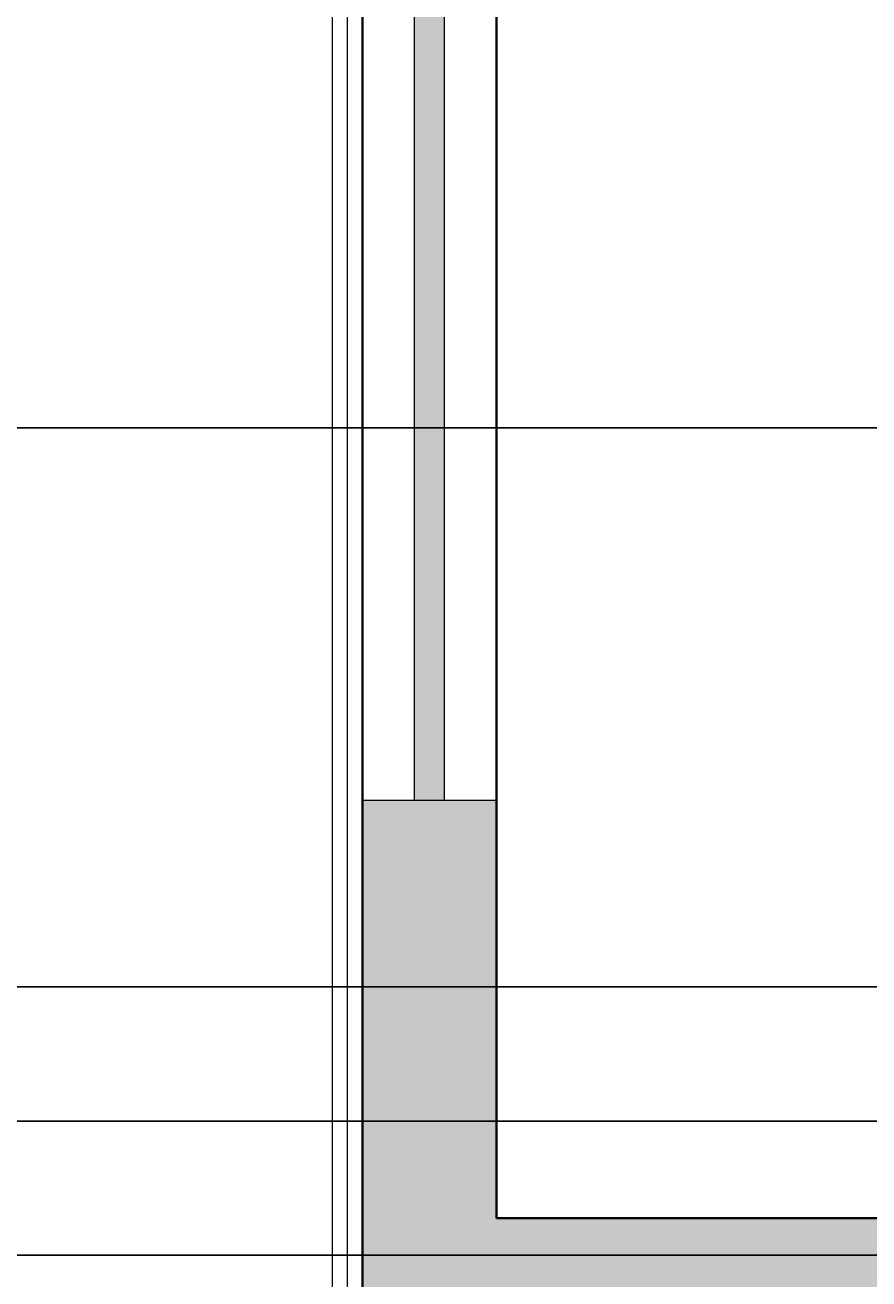
# Model space of a CAD drawing. Units: inches. Extents: x 311 to 815, y -527 to 136.
# Tile 7 of 21: x 388 to 444, y -294 to -210. Entities that reach past the tile are written whole.
import ezdxf

# ---------------------------------------------------------------- set-up
doc = ezdxf.new("R2010")
doc.units = ezdxf.units.IN
doc.header["$MEASUREMENT"] = 0
for name, color, linetype, lineweight in [('A-ANNO-DIMS', 1, 'Continuous', 18), ('A-FLOR-EDGE', 1, 'Continuous', 18), ('A-GLAZ-PATT', 5, 'Continuous', 13), ('A-WALL-PATT', 242, 'Continuous', 13), ('wall', 1, 'Continuous', 35), ('win', 5, 'Continuous', 18)]:
    doc.layers.add(name, color=color, linetype=linetype, lineweight=lineweight)
doc.styles.get("Standard").update_dxf_attribs({"font": 'arial.ttf'})
doc.dimstyles.get("Standard").update_dxf_attribs({"dimtxt": 0.18, "dimasz": 0.18, "dimexe": 0.18, "dimexo": 0.0625, "dimgap": 0.09, "dimtad": 0, "dimtih": 1, "dimtoh": 1, "dimdec": 1, "dimzin": 0, "dimdsep": 46, "dimlunit": 4, "dimtxsty": 'Standard', "dimcen": 0.09, "dimadec": 0, "dimazin": 0, "dimtfac": 1, "dimtdec": 1, "dimtofl": 0, "dimtmove": 0, "dimatfit": 3, "dimfxl": 1, "dimtolj": 1, "dimtzin": 0, "dimarcsym": 0})

# ---------------------------------------------------------------- blocks, each defined once
blk = doc.blocks.new('_ArchTick')
at = {"color": 0, "linetype": 'ByBlock', "const_width": 0.15}
blk.add_lwpolyline([(-0.5, -0.5), (0.5, 0.5)], dxfattribs=at)
blk = doc.blocks.new('_Oblique')
at = {"color": 0, "linetype": 'ByBlock', "lineweight": -2}
blk.add_line((-0.5, -0.5), (0.5, 0.5), dxfattribs=at)
blk = doc.blocks.new('*D3')
at = {"layer": 'A-ANNO-DIMS', "color": 0, "lineweight": -2, "transparency": 16777216}
for p, q in [((377.538, 21.872), (377.538, -221.609)), ((377.538, -482.128), (377.538, -238.646))]:
    blk.add_line(p, q, dxfattribs=at)
at = {"layer": 'Defpoints', "color": 0, "transparency": 16777216}
for p in [(410.323, 21.872), (377.538, -482.128), (410.323, -482.128)]:
    blk.add_point(p, dxfattribs=at)
at = {"layer": 'A-ANNO-DIMS', "color": 0, "lineweight": -2, "transparency": 16777216, "xscale": 9, "yscale": 9, "zscale": 9}
for name, p, rotation in [('_ArchTick', (377.538, 21.872), 90), ('_Oblique', (377.538, -482.128), 270)]:
    blk.add_blockref(name, p, dxfattribs=dict(at, rotation=rotation))
at = {"layer": 'A-ANNO-DIMS', "color": 0, "transparency": 16777216, "insert": (377.538, -230.128), "char_height": 9, "attachment_point": 5}
blk.add_mtext("\\A1;42'", dxfattribs=at)
blk = doc.blocks.new('WIN-60IN')
for p, q in [((9, 60), (0, 60)), ((3.5, 0), (3.5, 60)), ((5.5, 0), (5.5, 60)), ((9, 0), (0, 0))]:
    blk.add_line(p, q)
blk = doc.blocks.new('*D33')
at = {"layer": 'A-ANNO-DIMS', "color": 0, "lineweight": -2, "transparency": 16777216}
for p, q in [((609.26, -237.128), (377.793, -237.128)), ((377.973, -237.308), (377.973, -255.695)), ((377.973, -274.448), (377.973, -256.061)), ((609.26, -274.628), (377.793, -274.628))]:
    blk.add_line(p, q, dxfattribs=at)
at = {"layer": 'A-ANNO-DIMS', "color": 0, "transparency": 16777216}
for points in [[(377.943, -237.308), (378.003, -237.308), (377.973, -237.128)], [(377.943, -274.448), (378.003, -274.448), (377.973, -274.628)]]:
    blk.add_solid(points, dxfattribs=at)
at = {"layer": 'Defpoints', "color": 0, "transparency": 16777216}
for p in [(609.323, -237.128), (377.973, -274.628), (609.323, -274.628)]:
    blk.add_point(p, dxfattribs=at)
at = {"layer": 'A-ANNO-DIMS', "color": 0, "transparency": 16777216, "insert": (377.973, -255.878), "char_height": 0.18, "attachment_point": 5}
blk.add_mtext('\\A1;3\'-1 1/2"', dxfattribs=at)
blk = doc.blocks.new('*D36')
at = {"layer": 'A-ANNO-DIMS', "color": 0, "lineweight": -2, "transparency": 16777216}
for p, q in [((665.26, -283.628), (377.793, -283.628)), ((377.973, -283.808), (377.973, -287.946)), ((377.973, -292.448), (377.973, -288.31)), ((665.26, -292.628), (377.793, -292.628))]:
    blk.add_line(p, q, dxfattribs=at)
at = {"layer": 'A-ANNO-DIMS', "color": 0, "transparency": 16777216}
for points in [[(377.943, -283.808), (378.003, -283.808), (377.973, -283.628)], [(377.943, -292.448), (378.003, -292.448), (377.973, -292.628)]]:
    blk.add_solid(points, dxfattribs=at)
at = {"layer": 'Defpoints', "color": 0, "transparency": 16777216}
for p in [(665.323, -283.628), (377.973, -292.628), (665.323, -292.628)]:
    blk.add_point(p, dxfattribs=at)
at = {"layer": 'A-ANNO-DIMS', "color": 0, "transparency": 16777216, "insert": (377.973, -288.128), "char_height": 0.18, "attachment_point": 5}
blk.add_mtext('\\A1;0\'-9"', dxfattribs=at)

msp = doc.modelspace()

# ---------------------------------------------------------------- hatches: boundary and pattern name
at = {"layer": 'A-GLAZ-PATT'}
h = msp.add_hatch(color=256, dxfattribs=at)
h.dxf.hatch_style = 1
h.paths.add_polyline_path([(415.823, -202.128), (413.823, -202.128), (413.823, -262.128), (415.823, -262.128)])
h.paths.add_polyline_path([(415.823, -390.84), (413.823, -390.84), (413.823, -450.84), (415.823, -450.84)])
h.paths.add_polyline_path([(415.823, -311.568), (413.823, -311.568), (413.823, -335.568), (415.823, -335.568)])
h.paths.add_polyline_path([(509.323, -476.628), (449.323, -476.628), (449.323, -478.628), (509.323, -478.628)])
h.paths.add_polyline_path([(606.823, -476.628), (582.823, -476.628), (582.823, -478.628), (606.823, -478.628)])
h.paths.add_polyline_path([(678.823, -476.628), (654.823, -476.628), (654.823, -478.628), (678.823, -478.628)])
h.paths.add_polyline_path([(718.823, -385.128), (716.823, -385.128), (716.823, -445.128), (718.823, -445.128)])
h.paths.add_polyline_path([(718.823, -262.628), (716.823, -262.628), (716.823, -322.628), (718.823, -322.628)])
h.paths.add_polyline_path([(718.823, -140.128), (716.823, -140.128), (716.823, -200.128), (718.823, -200.128)])
h.paths.add_polyline_path([(718.823, -18.128), (716.823, -18.128), (716.823, -42.128), (718.823, -42.128)])
h.paths.add_polyline_path([(686.823, 18.372), (626.823, 18.372), (626.823, 16.372), (686.823, 16.372)])
h.paths.add_polyline_path([(581.823, 18.372), (557.823, 18.372), (557.823, 16.372), (581.823, 16.372)])
h.paths.add_polyline_path([(509.323, 18.372), (449.323, 18.372), (449.323, 16.372), (509.323, 16.372)])
at = {"layer": 'A-WALL-PATT'}
h = msp.add_hatch(color=256, dxfattribs=at)
h.dxf.hatch_style = 1
h.paths.add_polyline_path([(557.823, 21.872), (509.323, 21.872), (509.323, 12.872), (539.323, 12.872), (539.323, -112.128), (548.323, -112.128), (548.323, -58.628), (557.823, -58.628), (557.823, -49.628), (548.323, -49.628), (548.323, 12.872), (557.823, 12.872)])
h.paths.add_polyline_path([(449.323, 21.872), (410.323, 21.872), (410.323, -15.128), (419.323, -15.128), (419.323, 12.872), (449.323, 12.872)])
h.paths.add_polyline_path([(626.823, 21.872), (581.823, 21.872), (581.823, 12.872), (591.323, 12.872), (591.323, -49.628), (581.823, -49.628), (581.823, -58.628), (591.323, -58.628), (591.323, -112.128), (600.323, -112.128), (600.323, 12.872), (626.823, 12.872)])
h.paths.add_polyline_path([(722.323, 21.872), (686.823, 21.872), (686.823, 12.872), (713.323, 12.872), (713.323, -18.128), (722.323, -18.128)])
h.paths.add_polyline_path([(722.323, -42.128), (713.323, -42.128), (713.323, -73.128), (722.323, -73.128)])
h.paths.add_polyline_path([(501.323, -103.128), (419.323, -103.128), (419.323, -75.128), (410.323, -75.128), (410.323, -126.628), (419.323, -126.628), (419.323, -112.128), (492.323, -112.128), (492.323, -143.128), (501.323, -143.128)])
h.paths.add_polyline_path([(548.323, -165.128), (419.323, -165.128), (419.323, -150.628), (410.323, -150.628), (410.323, -202.128), (419.323, -202.128), (419.323, -174.128), (548.323, -174.128)])
h.paths.add_polyline_path([(722.323, -103.128), (636.323, -103.128), (636.323, -112.128), (713.323, -112.128), (713.323, -140.128), (722.323, -140.128)])
h.paths.add_polyline_path([(548.323, -210.128), (539.323, -210.128), (539.323, -290.128), (419.323, -290.128), (419.323, -262.128), (410.323, -262.128), (410.323, -311.568), (419.323, -311.568), (419.323, -299.128), (469.323, -299.128), (469.323, -348.128), (443.323, -348.128), (443.323, -357.128), (478.323, -357.128), (478.323, -299.128), (548.323, -299.128)])
h.paths.add_polyline_path([(722.323, -200.128), (713.323, -200.128), (713.323, -228.128), (609.323, -228.128), (609.323, -237.128), (713.323, -237.128), (713.323, -262.628), (722.323, -262.628)])
h.paths.add_polyline_path([(722.323, -322.628), (713.323, -322.628), (713.323, -348.128), (633.323, -348.128), (633.323, -357.128), (713.323, -357.128), (713.323, -385.128), (722.323, -385.128)])
h.paths.add_polyline_path([(419.323, -335.568), (410.323, -335.568), (410.323, -390.84), (419.323, -390.84)])
h.paths.add_polyline_path([(419.323, -450.84), (410.323, -450.84), (410.323, -482.128), (449.323, -482.128), (449.323, -473.128), (419.323, -473.128)])
h.paths.add_polyline_path([(582.823, -473.128), (548.323, -473.128), (548.323, -348.128), (539.323, -348.128), (539.323, -473.128), (509.323, -473.128), (509.323, -482.128), (582.823, -482.128)])
h.paths.add_polyline_path([(722.323, -445.128), (713.323, -445.128), (713.323, -473.128), (678.823, -473.128), (678.823, -482.128), (722.323, -482.128)])

# ---------------------------------------------------------------- linework, layer by layer
at = {"layer": 'A-FLOR-EDGE'}
for p, q in [((408.323, -484.128), (408.323, 23.872)), ((409.323, -483.128), (409.323, 22.872))]:
    msp.add_line(p, q, dxfattribs=at)
at = {"layer": 'wall'}
for p, q in [((410.323, -482.128), (410.323, 21.872)), ((419.323, -290.128), (419.323, -174.128)), ((539.323, -290.128), (419.323, -290.128))]:
    msp.add_line(p, q, dxfattribs=at)

# ---------------------------------------------------------------- block references
at = {"layer": 'win'}
msp.add_blockref('WIN-60IN', (410.323, -262.128), dxfattribs=at)

# ---------------------------------------------------------------- dimensions: what is measured, and where the dimension line sits
at = {"layer": 'A-ANNO-DIMS'}
for base, p1, p2, override, picture, middle in [((377.538, -482.128), (410.323, 21.872), (410.323, -482.128), {"dimtxt": 9, "dimasz": 9, "dimgap": 4, "dimblk1": 'ArchTick', "dimblk2": 'Oblique', "dimsah": 1, "dimse1": 1, "dimse2": 1, "dimclrd": 0, "dimclre": 0, "dimclrt": 0}, '*D3', (377.538, -230.128)), ((377.973, -274.628), (609.323, -237.128), (609.323, -274.628), {"dimdec": 1, "dimlfac": 1, "dimrnd": 0, "dimzin": 1, "dimdsep": 46, "dimlunit": 4, "dimfrac": 2}, '*D33', (377.973, -255.878)), ((377.973, -292.628), (665.323, -283.628), (665.323, -292.628), {"dimdec": 1, "dimlfac": 1, "dimrnd": 0, "dimzin": 1, "dimdsep": 46, "dimlunit": 4, "dimfrac": 2}, '*D36', (377.973, -288.128))]:
    dim = msp.add_linear_dim(base=base, p1=p1, p2=p2, angle=90, dimstyle='Standard', override=override, dxfattribs=at)
    dim.commit()
    dim.dimension.update_dxf_attribs({"geometry": picture, "text_midpoint": middle})

doc.saveas('drawing.dxf')
